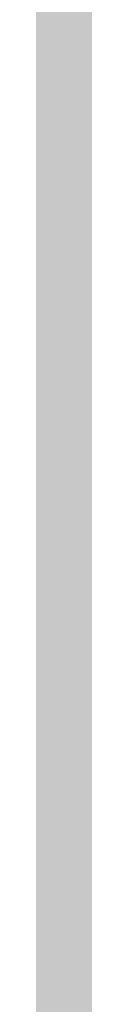
# Model space of a CAD drawing. Units: millimetres. Extents: x 0 to 2267, y 0 to 1823.
# Tile 41 of 256: x 1593.4369 to 1593.4507, y 1226.3857 to 1226.718. Entities that reach past the tile are written whole.
import ezdxf

# ---------------------------------------------------------------- set-up
doc = ezdxf.new("R2010")
doc.units = ezdxf.units.MM
doc.header["$MEASUREMENT"] = 0
doc.layers.add('M-HATC', color=252, linetype='Continuous', lineweight=18)

msp = doc.modelspace()

# ---------------------------------------------------------------- hatches: boundary and pattern name
at = {"layer": 'M-HATC'}
h = msp.add_hatch(color=256, dxfattribs=at)
h.dxf.hatch_style = 1
h.paths.add_polyline_path([(2055.77105, 1603.06204), (1381.08677, 1603.06204), (1381.08677, 1598.06204), (2055.77105, 1598.06204)])
h.paths.add_polyline_path([(2055.77105, 1598.06204), (1381.08677, 1598.06204), (1381.08677, 1593.06204), (2055.77105, 1593.06204)])
h.paths.add_polyline_path([(2051.30737, 1536.76088), (1385.55044, 1536.76088), (1385.55044, 1526.76088), (1387.55044, 1526.76088), (1388.53662, 1525.05276), (1385.33187, 1521.23348), (1385.33187, 1521.22256), (2050.25417, 1522.74913), (2048.32119, 1525.05276), (2049.30737, 1526.76088), (2051.30737, 1526.76088)])
edge = h.paths.add_edge_path()
edge.add_arc((1847.53451, 1379.14917), 135, 222.6030607, 222.8908505, ccw=False)
edge.add_line((1748.16629, 1287.76561), (1683.09212, 1287.76561))
edge.add_arc((1583.7239, 1379.14917), 135, 317.1091495, 317.3969393, ccw=False)
edge.add_arc((1678.9686, 1290.67067), 5, 222.89085, 317.10915, ccw=False)
edge.add_arc((1774.21331, 1379.14917), 135, 222.6030607, 222.8908505, ccw=False)
edge.add_line((1674.84509, 1287.76561), (1609.77092, 1287.76561))
edge.add_arc((1510.4027, 1379.14917), 135, 317.1091495, 317.3969393, ccw=False)
edge.add_arc((1605.6474, 1290.67067), 5, 222.89085, 317.10915, ccw=False)
edge.add_arc((1700.89211, 1379.14917), 135, 222.6030607, 222.8908505, ccw=False)
edge.add_line((1601.52388, 1287.76561), (1536.44972, 1287.76561))
edge.add_arc((1437.08149, 1379.14917), 135, 317.1091495, 317.3969393, ccw=False)
edge.add_arc((1532.3262, 1290.67067), 5, 222.89085, 317.10915, ccw=False)
edge.add_arc((1627.57091, 1379.14917), 135, 222.6030607, 222.8908505, ccw=False)
edge.add_line((1528.20268, 1287.76561), (1505.92891, 1287.76561))
edge.add_spline(control_points=[(1505.92891, 1287.76561), (1504.26224, 1287.76561), (1504.26224, 1282.76561), (1505.92891, 1282.76561)], knot_values=[0, 0, 0, 0, 5, 5, 5, 5], degree=3, periodic=0)
edge.add_line((1505.92891, 1282.76561), (1930.92891, 1282.76561))
edge.add_spline(control_points=[(1930.92891, 1282.76561), (1932.59557, 1282.76561), (1932.59557, 1287.76561), (1930.92891, 1287.76561)], knot_values=[0, 0, 0, 0, 5, 5, 5, 5], degree=3, periodic=0)
edge.add_line((1930.92891, 1287.76561), (1903.05573, 1287.76561))
edge.add_arc((1803.6875, 1379.14917), 135, 317.1091495, 317.3969393, ccw=False)
edge.add_arc((1898.93221, 1290.67067), 5, 222.89085, 317.10915, ccw=False)
edge.add_arc((1994.17691, 1379.14917), 135, 222.6030607, 222.8908505, ccw=False)
edge.add_line((1894.80869, 1287.76561), (1829.73452, 1287.76561))
edge.add_arc((1730.3663, 1379.14917), 135, 317.1091495, 317.3969393, ccw=False)
edge.add_arc((1825.61101, 1290.67067), 5, 222.89085, 317.10915, ccw=False)
edge.add_arc((1920.85571, 1379.14917), 135, 222.6030607, 222.8908505, ccw=False)
edge.add_line((1821.48749, 1287.76561), (1756.41332, 1287.76561))
edge.add_arc((1657.0451, 1379.14917), 135, 317.1091495, 317.3969393, ccw=False)
edge.add_arc((1752.28981, 1290.67067), 5, 222.89085, 317.10915, ccw=False)
edge = h.paths.add_edge_path()
edge.add_spline(control_points=[(1843.42891, 1227.24746), (1845.09557, 1227.24746), (1845.09557, 1232.24746), (1843.42891, 1232.24746)], knot_values=[0, 0, 0, 0, 5, 5, 5, 5], degree=3, periodic=0)
edge.add_line((1843.42891, 1232.24746), (1593.42891, 1232.24746))
edge.add_spline(control_points=[(1593.42891, 1232.24746), (1591.76224, 1232.24746), (1591.76224, 1227.24746), (1593.42891, 1227.24746)], knot_values=[0, 0, 0, 0, 5, 5, 5, 5], degree=3, periodic=0)
edge.add_line((1593.42891, 1227.24746), (1843.42891, 1227.24746))
h.paths.add_polyline_path([(1905.92891, 1127.41706), (1530.92891, 1127.41706, 0.414214), (1520.92891, 1117.41706), (1530.92891, 1117.41706), (1915.92891, 1117.41706, 0.414214)])
edge = h.paths.add_edge_path()
edge.add_arc((1397.08577, 1498.40775), 12.72993, 90.782146, 190.878706, ccw=False)
edge.add_line((1396.912, 1511.13649), (1428.00968, 1511.34875))
edge.add_line((1428.00968, 1511.34875), (1433.00968, 1511.34875))
edge.add_line((1433.00968, 1511.34875), (1434.439, 1511.34875))
edge.add_arc((1419.474, 1498.08041), 20, 41.560995, 74.082109)
edge.add_line((1424.95919, 1517.31353), (1399.93509, 1517.25608))
edge.add_spline(control_points=[(1399.93074, 1517.25607), (1399.88398, 1517.21312), (1399.8328, 1517.16893), (1399.77741, 1517.1236)], knot_values=[11.567499, 11.567499, 11.567499, 11.567499, 11.814249, 11.814249, 11.814249, 11.814249], degree=3, periodic=0)
edge.add_spline(control_points=[(1399.63279, 1517.00986), (1399.58305, 1516.97214), (1399.53072, 1516.93375), (1399.47591, 1516.89474)], knot_values=[11.167718, 11.167718, 11.167718, 11.167718, 11.365188, 11.365188, 11.365188, 11.365188], degree=3, periodic=0)
edge.add_spline(control_points=[(1399.33981, 1516.80007), (1399.15144, 1516.67185), (1398.93836, 1516.5377), (1398.70404, 1516.39942)], knot_values=[10.376405, 10.376405, 10.376405, 10.376405, 11.00994, 11.00994, 11.00994, 11.00994], degree=3, periodic=0)
edge.add_spline(control_points=[(1398.65716, 1516.37187), (1398.57885, 1516.32602), (1398.49825, 1516.27974), (1398.41549, 1516.23309)], knot_values=[10.125175, 10.125175, 10.125175, 10.125175, 10.334406, 10.334406, 10.334406, 10.334406], degree=3, periodic=0)
edge.add_spline(control_points=[(1398.26422, 1516.14874), (1398.19595, 1516.11107), (1398.12634, 1516.07319), (1398.05546, 1516.03513)], knot_values=[9.832246, 9.832246, 9.832246, 9.832246, 9.999658, 9.999658, 9.999658, 9.999658], degree=3, periodic=0)
edge.add_spline(control_points=[(1397.9987, 1516.00476), (1397.73115, 1515.86211), (1397.44602, 1515.71707), (1397.14664, 1515.57138)], knot_values=[9.161808, 9.161808, 9.161808, 9.161808, 9.787769, 9.787769, 9.787769, 9.787769], degree=3, periodic=0)
edge.add_spline(control_points=[(1397.14664, 1515.57138), (1396.84182, 1515.42305), (1396.52223, 1515.27404), (1396.1914, 1515.12621)], knot_values=[8.524455, 8.524455, 8.524455, 8.524455, 9.161808, 9.161808, 9.161808, 9.161808], degree=3, periodic=0)
edge.add_spline(control_points=[(1396.07771, 1515.07565), (1395.98538, 1515.03478), (1395.89222, 1514.99402), (1395.7983, 1514.9534)], knot_values=[8.275193, 8.275193, 8.275193, 8.275193, 8.451726, 8.451726, 8.451726, 8.451726], degree=3, periodic=0)
edge.add_spline(control_points=[(1395.60184, 1514.86912), (1395.49975, 1514.82568), (1395.39685, 1514.78244), (1395.29322, 1514.73944)], knot_values=[7.962917, 7.962917, 7.962917, 7.962917, 8.152764, 8.152764, 8.152764, 8.152764], degree=3, periodic=0)
edge.add_spline(control_points=[(1395.21158, 1514.70568), (1394.82779, 1514.5475), (1394.43452, 1514.39287), (1394.03645, 1514.24422)], knot_values=[7.21254, 7.21254, 7.21254, 7.21254, 7.913148, 7.913148, 7.913148, 7.913148], degree=3, periodic=0)
edge.add_spline(control_points=[(1394.03645, 1514.24422), (1393.70758, 1514.12142), (1393.37544, 1514.0027), (1393.04267, 1513.88945)], knot_values=[6.633733, 6.633733, 6.633733, 6.633733, 7.21254, 7.21254, 7.21254, 7.21254], degree=3, periodic=0)
edge.add_spline(control_points=[(1392.82142, 1513.81499), (1392.71978, 1513.78118), (1392.61815, 1513.74791), (1392.51658, 1513.71521)], knot_values=[6.328796, 6.328796, 6.328796, 6.328796, 6.505493, 6.505493, 6.505493, 6.505493], degree=3, periodic=0)
edge.add_spline(control_points=[(1392.51658, 1513.71521), (1392.31873, 1513.65151), (1392.12116, 1513.59001), (1391.92441, 1513.53098)], knot_values=[5.984605, 5.984605, 5.984605, 5.984605, 6.328796, 6.328796, 6.328796, 6.328796], degree=3, periodic=0)
edge.add_spline(control_points=[(1391.79155, 1513.49146), (1391.31215, 1513.35011), (1390.83842, 1513.22392), (1390.37844, 1513.11711)], knot_values=[5.066697, 5.066697, 5.066697, 5.066697, 5.907055, 5.907055, 5.907055, 5.907055], degree=3, periodic=0)
edge.add_spline(control_points=[(1390.37844, 1513.11711), (1390.17973, 1513.07097), (1389.98359, 1513.02845), (1389.79067, 1512.98988)], knot_values=[4.70367, 4.70367, 4.70367, 4.70367, 5.066695, 5.066695, 5.066695, 5.066695], degree=3, periodic=0)
edge.add_spline(control_points=[(1389.42203, 1512.92036), (1389.24588, 1512.88922), (1389.0729, 1512.86172), (1388.90364, 1512.83814)], knot_values=[4.130571, 4.130571, 4.130571, 4.130571, 4.469816, 4.469816, 4.469816, 4.469816], degree=3, periodic=0)
edge.add_spline(control_points=[(1388.90364, 1512.83814), (1388.59103, 1512.7946), (1388.29108, 1512.76444), (1388.00714, 1512.74941)], knot_values=[3.504031, 3.504031, 3.504031, 3.504031, 4.130571, 4.130571, 4.130571, 4.130571], degree=3, periodic=0)
edge.add_spline(control_points=[(1387.9356, 1512.74593), (1387.85378, 1512.74231), (1387.77334, 1512.73997), (1387.69435, 1512.73898)], knot_values=[3.268866, 3.268866, 3.268866, 3.268866, 3.451164, 3.451164, 3.451164, 3.451164], degree=3, periodic=0)
edge.add_spline(control_points=[(1387.33512, 1512.74426), (1387.20757, 1512.74991), (1387.08472, 1512.7597), (1386.96699, 1512.77385)], knot_values=[2.670686, 2.670686, 2.670686, 2.670686, 2.984, 2.984, 2.984, 2.984], degree=3, periodic=0)
edge.add_spline(control_points=[(1386.83274, 1512.79225), (1386.82093, 1512.79407), (1386.80917, 1512.79594), (1386.79747, 1512.79787)], knot_values=[2.516981, 2.516981, 2.516981, 2.516981, 2.549528, 2.549528, 2.549528, 2.549528], degree=3, periodic=0)
edge.add_spline(control_points=[(1386.45257, 1512.87348), (1386.42573, 1512.88105), (1386.39931, 1512.88895), (1386.3733, 1512.89719)], knot_values=[2.095869, 2.095869, 2.095869, 2.095869, 2.17941, 2.17941, 2.17941, 2.17941], degree=3, periodic=0)
edge.add_spline(control_points=[(1386.06911, 1513.01889), (1386.06338, 1513.02174), (1386.05768, 1513.02463), (1386.05201, 1513.02753)], knot_values=[1.72453, 1.72453, 1.72453, 1.72453, 1.745933, 1.745933, 1.745933, 1.745933], degree=3, periodic=0)
edge.add_arc((1399.474, 1498.08041), 20, 131.824322, 180)
edge.add_arc((1630.33362, 1505.54843), 250.97076, 181.7051759, 236.427975)
edge.add_arc((1605.33992, 1483.30441), 218.7822, 238.660829, 243.3496099)
edge.add_arc((1647.09105, 1510.35917), 262.89859, 183.1298361, 237.8534422, ccw=False)
h.paths.add_polyline_path([(1406.53685, 1391.96444, 0.149382), (1491.55061, 1296.44177, -0.129517)], flags=17)
edge = h.paths.add_edge_path()
edge.add_arc((2037.38381, 1498.08041), 20, 0, 48.265868)
edge.add_spline(control_points=[(2050.69731, 1513.00525), (2050.65121, 1512.98471), (2050.60338, 1512.96554), (2050.55388, 1512.94771)], knot_values=[1.835652, 1.835652, 1.835652, 1.835652, 2.000781, 2.000781, 2.000781, 2.000781], degree=3, periodic=0)
edge.add_spline(control_points=[(2050.46156, 1512.91661), (2050.479, 1512.9221), (2050.49625, 1512.92774), (2050.51332, 1512.93353)], knot_values=[2.045477, 2.045477, 2.045477, 2.045477, 2.101389, 2.101389, 2.101389, 2.101389], degree=3, periodic=0)
edge.add_spline(control_points=[(2050.12896, 1512.83416), (2050.19843, 1512.84734), (2050.26573, 1512.86233), (2050.33075, 1512.87919)], knot_values=[2.237629, 2.237629, 2.237629, 2.237629, 2.435841, 2.435841, 2.435841, 2.435841], degree=3, periodic=0)
edge.add_spline(control_points=[(2050.09463, 1512.82783), (2050.10613, 1512.82989), (2050.11757, 1512.832), (2050.12896, 1512.83416)], knot_values=[2.435841, 2.435841, 2.435841, 2.435841, 2.468321, 2.468321, 2.468321, 2.468321], degree=3, periodic=0)
edge.add_spline(control_points=[(2049.78433, 1512.78511), (2049.85521, 1512.79219), (2049.92435, 1512.80077), (2049.99166, 1512.81088)], knot_values=[2.563852, 2.563852, 2.563852, 2.563852, 2.748541, 2.748541, 2.748541, 2.748541], degree=3, periodic=0)
edge.add_spline(control_points=[(2049.4052, 1512.76169), (2049.5364, 1512.76526), (2049.66292, 1512.77299), (2049.78433, 1512.78511)], knot_values=[2.748541, 2.748541, 2.748541, 2.748541, 3.064882, 3.064882, 3.064882, 3.064882], degree=3, periodic=0)
edge.add_spline(control_points=[(2049.16976, 1512.75968), (2049.23364, 1512.7591), (2049.29654, 1512.7594), (2049.35844, 1512.7606)], knot_values=[3.102309, 3.102309, 3.102309, 3.102309, 3.2503, 3.2503, 3.2503, 3.2503], degree=3, periodic=0)
edge.add_spline(control_points=[(2048.85727, 1512.76911), (2048.96378, 1512.76378), (2049.068, 1512.76061), (2049.16976, 1512.75968)], knot_values=[3.2503, 3.2503, 3.2503, 3.2503, 3.486069, 3.486069, 3.486069, 3.486069], degree=3, periodic=0)
edge.add_spline(control_points=[(2048.69241, 1512.77892), (2048.3729, 1512.80093), (2048.0345, 1512.84106), (2047.68175, 1512.89697)], knot_values=[3.606429, 3.606429, 3.606429, 3.606429, 4.2989, 4.2989, 4.2989, 4.2989], degree=3, periodic=0)
edge.add_spline(control_points=[(2047.68175, 1512.89697), (2047.5458, 1512.91852), (2047.40772, 1512.94241), (2047.26776, 1512.96851)], knot_values=[4.2989, 4.2989, 4.2989, 4.2989, 4.565769, 4.565769, 4.565769, 4.565769], degree=3, periodic=0)
edge.add_spline(control_points=[(2047.26776, 1512.96851), (2047.14494, 1512.99141), (2047.02067, 1513.01601), (2046.89514, 1513.04223)], knot_values=[4.565769, 4.565769, 4.565769, 4.565769, 4.799971, 4.799971, 4.799971, 4.799971], degree=3, periodic=0)
edge.add_spline(control_points=[(2046.89514, 1513.04223), (2046.52865, 1513.11875), (2046.15135, 1513.20899), (2045.7676, 1513.31068)], knot_values=[4.799971, 4.799971, 4.799971, 4.799971, 5.483718, 5.483718, 5.483718, 5.483718], degree=3, periodic=0)
edge.add_spline(control_points=[(2045.7676, 1513.31068), (2045.3724, 1513.41539), (2044.97036, 1513.53225), (2044.56625, 1513.65876)], knot_values=[5.483718, 5.483718, 5.483718, 5.483718, 6.187866, 6.187866, 6.187866, 6.187866], degree=3, periodic=0)
edge.add_spline(control_points=[(2044.56625, 1513.65876), (2044.41491, 1513.70614), (2044.26329, 1513.75487), (2044.11163, 1513.80482)], knot_values=[6.187866, 6.187866, 6.187866, 6.187866, 6.451551, 6.451551, 6.451551, 6.451551], degree=3, periodic=0)
edge.add_spline(control_points=[(2044.11163, 1513.80482), (2043.99666, 1513.84269), (2043.88167, 1513.88126), (2043.76676, 1513.92048)], knot_values=[6.451551, 6.451551, 6.451551, 6.451551, 6.651434, 6.651434, 6.651434, 6.651434], degree=3, periodic=0)
edge.add_spline(control_points=[(2043.76676, 1513.92048), (2043.37157, 1514.05536), (2042.97738, 1514.19789), (2042.58863, 1514.34575)], knot_values=[6.651434, 6.651434, 6.651434, 6.651434, 7.338879, 7.338879, 7.338879, 7.338879], degree=3, periodic=0)
edge.add_spline(control_points=[(2042.58863, 1514.34575), (2042.16431, 1514.50715), (2041.74647, 1514.67491), (2041.34086, 1514.84603)], knot_values=[7.338879, 7.338879, 7.338879, 7.338879, 8.089209, 8.089209, 8.089209, 8.089209], degree=3, periodic=0)
edge.add_spline(control_points=[(2041.34086, 1514.84603), (2041.1028, 1514.94647), (2040.86896, 1515.04806), (2040.64049, 1515.1502)], knot_values=[8.089209, 8.089209, 8.089209, 8.089209, 8.529587, 8.529587, 8.529587, 8.529587], degree=3, periodic=0)
edge.add_spline(control_points=[(2040.50999, 1515.20887), (2040.08238, 1515.40218), (2039.67475, 1515.59705), (2039.29495, 1515.78939)], knot_values=[8.613818, 8.613818, 8.613818, 8.613818, 9.44571, 9.44571, 9.44571, 9.44571], degree=3, periodic=0)
edge.add_spline(control_points=[(2039.29495, 1515.78939), (2039.0618, 1515.90746), (2038.83914, 1516.02458), (2038.62878, 1516.1398)], knot_values=[9.44571, 9.44571, 9.44571, 9.44571, 9.956404, 9.956404, 9.956404, 9.956404], degree=3, periodic=0)
edge.add_spline(control_points=[(2038.62878, 1516.1398), (2038.51874, 1516.20007), (2038.41207, 1516.25982), (2038.30903, 1516.31891)], knot_values=[9.956404, 9.956404, 9.956404, 9.956404, 10.223542, 10.223542, 10.223542, 10.223542], degree=3, periodic=0)
edge.add_spline(control_points=[(2038.30903, 1516.31891), (2038.21377, 1516.37354), (2038.12161, 1516.42762), (2038.03275, 1516.48102)], knot_values=[10.223542, 10.223542, 10.223542, 10.223542, 10.47051, 10.47051, 10.47051, 10.47051], degree=3, periodic=0)
edge.add_spline(control_points=[(2038.03275, 1516.48102), (2037.78552, 1516.62961), (2037.56388, 1516.77304), (2037.37225, 1516.909)], knot_values=[10.47051, 10.47051, 10.47051, 10.47051, 11.15767, 11.15767, 11.15767, 11.15767], degree=3, periodic=0)
edge.add_spline(control_points=[(2037.37225, 1516.909), (2037.27893, 1516.9752), (2037.19274, 1517.03963), (2037.11417, 1517.10203)], knot_values=[11.15767, 11.15767, 11.15767, 11.15767, 11.49227, 11.49227, 11.49227, 11.49227], degree=3, periodic=0)
edge.add_spline(control_points=[(2036.85638, 1517.32585), (2036.91481, 1517.26923), (2036.98143, 1517.21027), (2037.05573, 1517.14922)], knot_values=[11.577341, 11.577341, 11.577341, 11.577341, 11.91035, 11.91035, 11.91035, 11.91035], degree=3, periodic=0)
edge.add_spline(control_points=[(2036.80739, 1517.37475), (2036.82301, 1517.35865), (2036.83935, 1517.34235), (2036.85638, 1517.32585)], knot_values=[11.91035, 11.91035, 11.91035, 11.91035, 12.007402, 12.007402, 12.007402, 12.007402], degree=3, periodic=0)
edge.add_spline(control_points=[(2036.70167, 1517.494), (2036.71042, 1517.48299), (2036.71958, 1517.47185), (2036.72913, 1517.4606)], knot_values=[12.184155, 12.184155, 12.184155, 12.184155, 12.255409, 12.255409, 12.255409, 12.255409], degree=3, periodic=0)
edge.add_spline(control_points=[(2036.6159, 1517.6205), (2036.61998, 1517.61304), (2036.6243, 1517.6055), (2036.62885, 1517.59789)], knot_values=[12.487913, 12.487913, 12.487913, 12.487913, 12.541035, 12.541035, 12.541035, 12.541035], degree=3, periodic=0)
edge.add_spline(control_points=[(2036.56349, 1517.78599), (2036.56372, 1517.77936), (2036.56423, 1517.77264), (2036.56502, 1517.76582)], knot_values=[12.911761, 12.911761, 12.911761, 12.911761, 12.968286, 12.968286, 12.968286, 12.968286], degree=3, periodic=0)
edge.add_spline(control_points=[(2036.61663, 1517.93042), (2036.61248, 1517.92586), (2036.60857, 1517.92121), (2036.60491, 1517.91648)], knot_values=[13.382527, 13.382527, 13.382527, 13.382527, 13.433791, 13.433791, 13.433791, 13.433791], degree=3, periodic=0)
edge.add_spline(control_points=[(2036.74902, 1518.01695), (2036.73613, 1518.0116), (2036.72393, 1518.00601), (2036.71242, 1518.00018)], knot_values=[13.726299, 13.726299, 13.726299, 13.726299, 13.809928, 13.809928, 13.809928, 13.809928], degree=3, periodic=0)
edge.add_spline(control_points=[(2036.86043, 1518.05285), (2036.83863, 1518.04743), (2036.81809, 1518.04156), (2036.79879, 1518.03526)], knot_values=[13.910887, 13.910887, 13.910887, 13.910887, 14.02153, 14.02153, 14.02153, 14.02153], degree=3, periodic=0)
edge.add_line((2036.96387, 1518.08041), (2032.38381, 1518.08041))
edge.add_line((2032.38381, 1518.08041), (2027.38381, 1518.08041))
edge.add_line((2027.38381, 1518.08041), (2022.38381, 1518.08041))
edge.add_line((2022.38381, 1518.08041), (2017.38381, 1518.08041))
edge.add_arc((2017.38381, 1498.08041), 20, 90, 138.439005)
edge.add_line((2002.41881, 1511.34875), (2003.84813, 1511.34875))
edge.add_line((2003.84813, 1511.34875), (2008.84813, 1511.34875))
edge.add_line((2008.84813, 1511.34875), (2039.77204, 1511.13768))
edge.add_arc((2039.77204, 1498.40775), 12.72993, -10.878706, 90, ccw=False)
edge.add_arc((1789.76676, 1510.35917), 262.89859, 302.1465578, 356.8701639, ccw=False)
edge.add_arc((1831.51789, 1483.30441), 218.7822, 296.6503901, 301.339171)
edge.add_arc((1806.52419, 1505.54843), 250.97076, 303.572025, 358.2948241)
h.paths.add_polyline_path([(2030.32096, 1391.96444, -0.129517), (1945.3072, 1296.44177, 0.149382)], flags=17)
edge = h.paths.add_edge_path()
edge.add_spline(control_points=[(2037.2464, 1518.08209), (2037.28977, 1518.08098), (2037.33555, 1518.08041), (2037.3838, 1518.08041)], knot_values=[0.000012, 0.000012, 0.000012, 0.000012, 0.144754, 0.144754, 0.144754, 0.144754], degree=3, periodic=0)
edge.add_line((2037.33571, 1518.08041), (2037.00963, 1518.08041))
edge.add_spline(control_points=[(2037.00963, 1518.08041), (2036.98217, 1518.07678), (2036.95605, 1518.07266), (2036.93124, 1518.06808)], knot_values=[14.13465, 14.13465, 14.13465, 14.13465, 14.247197, 14.247197, 14.247197, 14.247197], degree=3, periodic=0)
edge.add_spline(control_points=[(2036.93124, 1518.06808), (2036.92764, 1518.06741), (2036.92407, 1518.06674), (2036.92053, 1518.06605)], knot_values=[14.118315, 14.118315, 14.118315, 14.118315, 14.13465, 14.13465, 14.13465, 14.13465], degree=3, periodic=0)
edge.add_spline(control_points=[(2036.92053, 1518.06605), (2036.9118, 1518.06436), (2036.90323, 1518.06262), (2036.89484, 1518.06081)], knot_values=[14.078086, 14.078086, 14.078086, 14.078086, 14.118315, 14.118315, 14.118315, 14.118315], degree=3, periodic=0)
edge.add_spline(control_points=[(2036.89484, 1518.06081), (2036.88304, 1518.05827), (2036.87157, 1518.05562), (2036.86043, 1518.05285)], knot_values=[14.02153, 14.02153, 14.02153, 14.02153, 14.078086, 14.078086, 14.078086, 14.078086], degree=3, periodic=0)
edge.add_spline(control_points=[(2036.86043, 1518.05285), (2036.83863, 1518.04743), (2036.81809, 1518.04156), (2036.79879, 1518.03526)], knot_values=[13.910887, 13.910887, 13.910887, 13.910887, 14.02153, 14.02153, 14.02153, 14.02153], degree=3, periodic=0)
edge.add_spline(control_points=[(2036.79879, 1518.03526), (2036.79809, 1518.03504), (2036.7974, 1518.03481), (2036.79671, 1518.03458)], knot_values=[13.906906, 13.906906, 13.906906, 13.906906, 13.910887, 13.910887, 13.910887, 13.910887], degree=3, periodic=0)
edge.add_spline(control_points=[(2036.79671, 1518.03458), (2036.78819, 1518.03178), (2036.77991, 1518.02888), (2036.77187, 1518.02591)], knot_values=[13.857826, 13.857826, 13.857826, 13.857826, 13.906906, 13.906906, 13.906906, 13.906906], degree=3, periodic=0)
edge.add_spline(control_points=[(2036.77187, 1518.02591), (2036.76402, 1518.023), (2036.75641, 1518.02002), (2036.74902, 1518.01695)], knot_values=[13.809928, 13.809928, 13.809928, 13.809928, 13.857826, 13.857826, 13.857826, 13.857826], degree=3, periodic=0)
edge.add_spline(control_points=[(2036.74902, 1518.01695), (2036.73613, 1518.0116), (2036.72393, 1518.00601), (2036.71242, 1518.00018)], knot_values=[13.726299, 13.726299, 13.726299, 13.726299, 13.809928, 13.809928, 13.809928, 13.809928], degree=3, periodic=0)
edge.add_spline(control_points=[(2036.71242, 1518.00018), (2036.71211, 1518.00002), (2036.71179, 1517.99986), (2036.71147, 1517.99969)], knot_values=[13.723993, 13.723993, 13.723993, 13.723993, 13.726299, 13.726299, 13.726299, 13.726299], degree=3, periodic=0)
edge.add_spline(control_points=[(2036.71147, 1517.99969), (2036.70634, 1517.99708), (2036.70134, 1517.99441), (2036.69648, 1517.9917)], knot_values=[13.686536, 13.686536, 13.686536, 13.686536, 13.723993, 13.723993, 13.723993, 13.723993], degree=3, periodic=0)
edge.add_spline(control_points=[(2036.69648, 1517.9917), (2036.6919, 1517.98914), (2036.68744, 1517.98654), (2036.6831, 1517.9839)], knot_values=[13.651251, 13.651251, 13.651251, 13.651251, 13.686536, 13.686536, 13.686536, 13.686536], degree=3, periodic=0)
edge.add_spline(control_points=[(2036.6831, 1517.9839), (2036.67641, 1517.97983), (2036.67001, 1517.97566), (2036.6639, 1517.97139)], knot_values=[13.596804, 13.596804, 13.596804, 13.596804, 13.651251, 13.651251, 13.651251, 13.651251], degree=3, periodic=0)
edge.add_spline(control_points=[(2036.6639, 1517.97139), (2036.66358, 1517.97117), (2036.66326, 1517.97094), (2036.66294, 1517.97072)], knot_values=[13.593956, 13.593956, 13.593956, 13.593956, 13.596804, 13.596804, 13.596804, 13.596804], degree=3, periodic=0)
edge.add_spline(control_points=[(2036.66294, 1517.97072), (2036.6603, 1517.96886), (2036.65771, 1517.96698), (2036.65518, 1517.96509)], knot_values=[13.570322, 13.570322, 13.570322, 13.570322, 13.593956, 13.593956, 13.593956, 13.593956], degree=3, periodic=0)
edge.add_spline(control_points=[(2036.65518, 1517.96509), (2036.65251, 1517.9631), (2036.64991, 1517.96108), (2036.64737, 1517.95905)], knot_values=[13.545477, 13.545477, 13.545477, 13.545477, 13.570322, 13.570322, 13.570322, 13.570322], degree=3, periodic=0)
edge.add_spline(control_points=[(2036.64737, 1517.95905), (2036.64721, 1517.95892), (2036.64705, 1517.9588), (2036.64689, 1517.95867)], knot_values=[13.543931, 13.543931, 13.543931, 13.543931, 13.545477, 13.545477, 13.545477, 13.545477], degree=3, periodic=0)
edge.add_spline(control_points=[(2036.64689, 1517.95867), (2036.64121, 1517.95411), (2036.63582, 1517.94945), (2036.63073, 1517.94468)], knot_values=[13.488237, 13.488237, 13.488237, 13.488237, 13.543931, 13.543931, 13.543931, 13.543931], degree=3, periodic=0)
edge.add_spline(control_points=[(2036.63073, 1517.94468), (2036.62817, 1517.94229), (2036.62569, 1517.93988), (2036.62329, 1517.93744)], knot_values=[13.460307, 13.460307, 13.460307, 13.460307, 13.488237, 13.488237, 13.488237, 13.488237], degree=3, periodic=0)
edge.add_spline(control_points=[(2036.62329, 1517.93744), (2036.62151, 1517.93564), (2036.61978, 1517.93383), (2036.61809, 1517.932)], knot_values=[13.439712, 13.439712, 13.439712, 13.439712, 13.460307, 13.460307, 13.460307, 13.460307], degree=3, periodic=0)
edge.add_spline(control_points=[(2036.61809, 1517.932), (2036.6176, 1517.93147), (2036.61711, 1517.93095), (2036.61663, 1517.93042)], knot_values=[13.433791, 13.433791, 13.433791, 13.433791, 13.439712, 13.439712, 13.439712, 13.439712], degree=3, periodic=0)
edge.add_spline(control_points=[(2036.61663, 1517.93042), (2036.61248, 1517.92586), (2036.60857, 1517.92121), (2036.60491, 1517.91648)], knot_values=[13.382527, 13.382527, 13.382527, 13.382527, 13.433791, 13.433791, 13.433791, 13.433791], degree=3, periodic=0)
edge.add_spline(control_points=[(2036.60491, 1517.91648), (2036.60258, 1517.91347), (2036.60036, 1517.91044), (2036.59824, 1517.90737)], knot_values=[13.350017, 13.350017, 13.350017, 13.350017, 13.382527, 13.382527, 13.382527, 13.382527], degree=3, periodic=0)
edge.add_spline(control_points=[(2036.59824, 1517.90737), (2036.59718, 1517.90585), (2036.59616, 1517.90433), (2036.59515, 1517.90279)], knot_values=[13.333922, 13.333922, 13.333922, 13.333922, 13.350017, 13.350017, 13.350017, 13.350017], degree=3, periodic=0)
edge.add_spline(control_points=[(2036.59515, 1517.90279), (2036.59452, 1517.90183), (2036.5939, 1517.90086), (2036.59329, 1517.89989)], knot_values=[13.323828, 13.323828, 13.323828, 13.323828, 13.333922, 13.333922, 13.333922, 13.333922], degree=3, periodic=0)
edge.add_spline(control_points=[(2036.59329, 1517.89989), (2036.59049, 1517.89545), (2036.5879, 1517.89094), (2036.5855, 1517.88637)], knot_values=[13.277545, 13.277545, 13.277545, 13.277545, 13.323828, 13.323828, 13.323828, 13.323828], degree=3, periodic=0)
edge.add_spline(control_points=[(2036.5855, 1517.88637), (2036.58355, 1517.88267), (2036.58174, 1517.87892), (2036.58006, 1517.87513)], knot_values=[13.240119, 13.240119, 13.240119, 13.240119, 13.277545, 13.277545, 13.277545, 13.277545], degree=3, periodic=0)
edge.add_spline(control_points=[(2036.58006, 1517.87513), (2036.57952, 1517.87393), (2036.579, 1517.87272), (2036.57849, 1517.87151)], knot_values=[13.228211, 13.228211, 13.228211, 13.228211, 13.240119, 13.240119, 13.240119, 13.240119], degree=3, periodic=0)
edge.add_spline(control_points=[(2036.57849, 1517.87151), (2036.57796, 1517.87023), (2036.57744, 1517.86896), (2036.57693, 1517.86767)], knot_values=[13.215717, 13.215717, 13.215717, 13.215717, 13.228211, 13.228211, 13.228211, 13.228211], degree=3, periodic=0)
edge.add_spline(control_points=[(2036.57693, 1517.86767), (2036.57548, 1517.86399), (2036.57414, 1517.86027), (2036.57293, 1517.85651)], knot_values=[13.179847, 13.179847, 13.179847, 13.179847, 13.215717, 13.215717, 13.215717, 13.215717], degree=3, periodic=0)
edge.add_spline(control_points=[(2036.57293, 1517.85651), (2036.5713, 1517.8515), (2036.56989, 1517.84641), (2036.56868, 1517.84126)], knot_values=[13.132017, 13.132017, 13.132017, 13.132017, 13.179847, 13.179847, 13.179847, 13.179847], degree=3, periodic=0)
edge.add_spline(control_points=[(2036.56868, 1517.84126), (2036.56844, 1517.84023), (2036.56821, 1517.8392), (2036.56798, 1517.83817)], knot_values=[13.122482, 13.122482, 13.122482, 13.122482, 13.132017, 13.132017, 13.132017, 13.132017], degree=3, periodic=0)
edge.add_spline(control_points=[(2036.56798, 1517.83817), (2036.56758, 1517.83634), (2036.56721, 1517.8345), (2036.56687, 1517.83266)], knot_values=[13.105592, 13.105592, 13.105592, 13.105592, 13.122482, 13.122482, 13.122482, 13.122482], degree=3, periodic=0)
edge.add_spline(control_points=[(2036.56687, 1517.83266), (2036.56622, 1517.82921), (2036.56567, 1517.82574), (2036.5652, 1517.82223)], knot_values=[13.074063, 13.074063, 13.074063, 13.074063, 13.105592, 13.105592, 13.105592, 13.105592], degree=3, periodic=0)
edge.add_spline(control_points=[(2036.5652, 1517.82223), (2036.5652, 1517.82223), (2036.5652, 1517.82223), (2036.5652, 1517.82223)], knot_values=[13.074043, 13.074043, 13.074043, 13.074043, 13.074063, 13.074063, 13.074063, 13.074063], degree=3, periodic=0)
edge.add_spline(control_points=[(2036.5652, 1517.82223), (2036.56443, 1517.81643), (2036.5639, 1517.81055), (2036.56361, 1517.8046)], knot_values=[13.021884, 13.021884, 13.021884, 13.021884, 13.074043, 13.074043, 13.074043, 13.074043], degree=3, periodic=0)
edge.add_spline(control_points=[(2036.56361, 1517.8046), (2036.56358, 1517.80401), (2036.56356, 1517.80342), (2036.56353, 1517.80283)], knot_values=[13.01674, 13.01674, 13.01674, 13.01674, 13.021884, 13.021884, 13.021884, 13.021884], degree=3, periodic=0)
edge.add_spline(control_points=[(2036.56353, 1517.80283), (2036.56344, 1517.80051), (2036.56338, 1517.79817), (2036.56336, 1517.79582)], knot_values=[12.996438, 12.996438, 12.996438, 12.996438, 13.01674, 13.01674, 13.01674, 13.01674], degree=3, periodic=0)
edge.add_spline(control_points=[(2036.56336, 1517.79582), (2036.56334, 1517.79257), (2036.56338, 1517.78929), (2036.56349, 1517.78599)], knot_values=[12.968286, 12.968286, 12.968286, 12.968286, 12.996438, 12.996438, 12.996438, 12.996438], degree=3, periodic=0)
edge.add_spline(control_points=[(2036.56349, 1517.78599), (2036.56372, 1517.77936), (2036.56423, 1517.77264), (2036.56502, 1517.76582)], knot_values=[12.911761, 12.911761, 12.911761, 12.911761, 12.968286, 12.968286, 12.968286, 12.968286], degree=3, periodic=0)
edge.add_spline(control_points=[(2036.56502, 1517.76582), (2036.56503, 1517.76573), (2036.56504, 1517.76564), (2036.56505, 1517.76555)], knot_values=[12.911017, 12.911017, 12.911017, 12.911017, 12.911761, 12.911761, 12.911761, 12.911761], degree=3, periodic=0)
edge.add_spline(control_points=[(2036.56505, 1517.76555), (2036.56541, 1517.76245), (2036.56583, 1517.75933), (2036.56631, 1517.75619)], knot_values=[12.88528, 12.88528, 12.88528, 12.88528, 12.911017, 12.911017, 12.911017, 12.911017], degree=3, periodic=0)
edge.add_spline(control_points=[(2036.56631, 1517.75619), (2036.56673, 1517.75341), (2036.5672, 1517.75062), (2036.56771, 1517.74782)], knot_values=[12.862519, 12.862519, 12.862519, 12.862519, 12.88528, 12.88528, 12.88528, 12.88528], degree=3, periodic=0)
edge.add_spline(control_points=[(2036.56771, 1517.74782), (2036.56779, 1517.74737), (2036.56788, 1517.74692), (2036.56796, 1517.74647)], knot_values=[12.858885, 12.858885, 12.858885, 12.858885, 12.862519, 12.862519, 12.862519, 12.862519], degree=3, periodic=0)
edge.add_spline(control_points=[(2036.56796, 1517.74647), (2036.5692, 1517.73986), (2036.57069, 1517.73316), (2036.57243, 1517.72638)], knot_values=[12.8053, 12.8053, 12.8053, 12.8053, 12.858885, 12.858885, 12.858885, 12.858885], degree=3, periodic=0)
edge.add_spline(control_points=[(2036.57243, 1517.72638), (2036.5734, 1517.72257), (2036.57446, 1517.71874), (2036.57559, 1517.71488)], knot_values=[12.775176, 12.775176, 12.775176, 12.775176, 12.8053, 12.8053, 12.8053, 12.8053], degree=3, periodic=0)
edge.add_spline(control_points=[(2036.57559, 1517.71488), (2036.57628, 1517.71252), (2036.577, 1517.71015), (2036.57775, 1517.70778)], knot_values=[12.756759, 12.756759, 12.756759, 12.756759, 12.775176, 12.775176, 12.775176, 12.775176], degree=3, periodic=0)
edge.add_spline(control_points=[(2036.57775, 1517.70778), (2036.57808, 1517.70674), (2036.57841, 1517.7057), (2036.57875, 1517.70466)], knot_values=[12.748742, 12.748742, 12.748742, 12.748742, 12.756759, 12.756759, 12.756759, 12.756759], degree=3, periodic=0)
edge.add_spline(control_points=[(2036.57875, 1517.70466), (2036.58082, 1517.6983), (2036.58309, 1517.69187), (2036.58557, 1517.68537)], knot_values=[12.69959, 12.69959, 12.69959, 12.69959, 12.748742, 12.748742, 12.748742, 12.748742], degree=3, periodic=0)
edge.add_spline(control_points=[(2036.58557, 1517.68537), (2036.58762, 1517.68001), (2036.5898, 1517.6746), (2036.59213, 1517.66916)], knot_values=[12.659038, 12.659038, 12.659038, 12.659038, 12.69959, 12.69959, 12.69959, 12.69959], degree=3, periodic=0)
edge.add_spline(control_points=[(2036.59213, 1517.66916), (2036.59397, 1517.66482), (2036.59591, 1517.66047), (2036.59793, 1517.65608)], knot_values=[12.626806, 12.626806, 12.626806, 12.626806, 12.659038, 12.659038, 12.659038, 12.659038], degree=3, periodic=0)
edge.add_spline(control_points=[(2036.59793, 1517.65608), (2036.59839, 1517.65507), (2036.59886, 1517.65406), (2036.59934, 1517.65305)], knot_values=[12.619394, 12.619394, 12.619394, 12.619394, 12.626806, 12.626806, 12.626806, 12.626806], degree=3, periodic=0)
edge.add_spline(control_points=[(2036.59934, 1517.65305), (2036.60435, 1517.64236), (2036.60987, 1517.63151), (2036.61589, 1517.6205)], knot_values=[12.541039, 12.541039, 12.541039, 12.541039, 12.619394, 12.619394, 12.619394, 12.619394], degree=3, periodic=0)
edge.add_spline(control_points=[(2036.61589, 1517.6205), (2036.61589, 1517.6205), (2036.6159, 1517.6205), (2036.6159, 1517.6205)], knot_values=[12.541035, 12.541035, 12.541035, 12.541035, 12.541039, 12.541039, 12.541039, 12.541039], degree=3, periodic=0)
edge.add_spline(control_points=[(2036.6159, 1517.6205), (2036.61998, 1517.61304), (2036.6243, 1517.6055), (2036.62885, 1517.59789)], knot_values=[12.487913, 12.487913, 12.487913, 12.487913, 12.541035, 12.541035, 12.541035, 12.541035], degree=3, periodic=0)
edge.add_spline(control_points=[(2036.62885, 1517.59789), (2036.63261, 1517.5916), (2036.63653, 1517.58526), (2036.64061, 1517.57888)], knot_values=[12.443982, 12.443982, 12.443982, 12.443982, 12.487913, 12.487913, 12.487913, 12.487913], degree=3, periodic=0)
edge.add_spline(control_points=[(2036.64061, 1517.57888), (2036.64144, 1517.57757), (2036.64228, 1517.57626), (2036.64313, 1517.57495)], knot_values=[12.434996, 12.434996, 12.434996, 12.434996, 12.443982, 12.443982, 12.443982, 12.443982], degree=3, periodic=0)
edge.add_spline(control_points=[(2036.64313, 1517.57495), (2036.65306, 1517.55958), (2036.66389, 1517.54394), (2036.6756, 1517.52803)], knot_values=[12.329647, 12.329647, 12.329647, 12.329647, 12.434996, 12.434996, 12.434996, 12.434996], degree=3, periodic=0)
edge.add_spline(control_points=[(2036.6756, 1517.52803), (2036.68385, 1517.51682), (2036.69254, 1517.50548), (2036.70167, 1517.494)], knot_values=[12.255409, 12.255409, 12.255409, 12.255409, 12.329647, 12.329647, 12.329647, 12.329647], degree=3, periodic=0)
edge.add_spline(control_points=[(2036.70167, 1517.494), (2036.71042, 1517.48299), (2036.71958, 1517.47185), (2036.72913, 1517.4606)], knot_values=[12.184155, 12.184155, 12.184155, 12.184155, 12.255409, 12.255409, 12.255409, 12.255409], degree=3, periodic=0)
edge.add_spline(control_points=[(2036.72913, 1517.4606), (2036.74363, 1517.44352), (2036.75904, 1517.42617), (2036.77534, 1517.40855)], knot_values=[12.075961, 12.075961, 12.075961, 12.075961, 12.184155, 12.184155, 12.184155, 12.184155], degree=3, periodic=0)
edge.add_spline(control_points=[(2036.77534, 1517.40855), (2036.77631, 1517.4075), (2036.77729, 1517.40645), (2036.77827, 1517.40539)], knot_values=[12.069502, 12.069502, 12.069502, 12.069502, 12.075961, 12.075961, 12.075961, 12.075961], degree=3, periodic=0)
edge.add_spline(control_points=[(2036.77827, 1517.40539), (2036.78768, 1517.39526), (2036.79739, 1517.38505), (2036.80739, 1517.37475)], knot_values=[12.007402, 12.007402, 12.007402, 12.007402, 12.069502, 12.069502, 12.069502, 12.069502], degree=3, periodic=0)
edge.add_spline(control_points=[(2036.80739, 1517.37475), (2036.82301, 1517.35865), (2036.83935, 1517.34235), (2036.85638, 1517.32585)], knot_values=[11.91035, 11.91035, 11.91035, 11.91035, 12.007402, 12.007402, 12.007402, 12.007402], degree=3, periodic=0)
edge.add_spline(control_points=[(2036.85638, 1517.32585), (2036.91481, 1517.26923), (2036.98143, 1517.21027), (2037.05573, 1517.14922)], knot_values=[11.577341, 11.577341, 11.577341, 11.577341, 11.91035, 11.91035, 11.91035, 11.91035], degree=3, periodic=0)
edge.add_spline(control_points=[(2037.05573, 1517.14922), (2037.07471, 1517.13362), (2037.0942, 1517.11789), (2037.11417, 1517.10203)], knot_values=[11.49227, 11.49227, 11.49227, 11.49227, 11.577341, 11.577341, 11.577341, 11.577341], degree=3, periodic=0)
edge.add_spline(control_points=[(2037.11417, 1517.10203), (2037.19274, 1517.03963), (2037.27893, 1516.9752), (2037.37225, 1516.909)], knot_values=[11.15767, 11.15767, 11.15767, 11.15767, 11.49227, 11.49227, 11.49227, 11.49227], degree=3, periodic=0)
edge.add_spline(control_points=[(2037.37225, 1516.909), (2037.56388, 1516.77304), (2037.78552, 1516.62961), (2038.03275, 1516.48102)], knot_values=[10.47051, 10.47051, 10.47051, 10.47051, 11.15767, 11.15767, 11.15767, 11.15767], degree=3, periodic=0)
edge.add_spline(control_points=[(2038.03275, 1516.48102), (2038.12161, 1516.42762), (2038.21377, 1516.37354), (2038.30903, 1516.31891)], knot_values=[10.223542, 10.223542, 10.223542, 10.223542, 10.47051, 10.47051, 10.47051, 10.47051], degree=3, periodic=0)
edge.add_spline(control_points=[(2038.30903, 1516.31891), (2038.41207, 1516.25982), (2038.51874, 1516.20007), (2038.62878, 1516.1398)], knot_values=[9.956404, 9.956404, 9.956404, 9.956404, 10.223542, 10.223542, 10.223542, 10.223542], degree=3, periodic=0)
edge.add_spline(control_points=[(2038.62878, 1516.1398), (2038.83914, 1516.02458), (2039.0618, 1515.90746), (2039.29495, 1515.78939)], knot_values=[9.44571, 9.44571, 9.44571, 9.44571, 9.956404, 9.956404, 9.956404, 9.956404], degree=3, periodic=0)
edge.add_spline(control_points=[(2039.29495, 1515.78939), (2039.67475, 1515.59705), (2040.08238, 1515.40218), (2040.50999, 1515.20887)], knot_values=[8.613818, 8.613818, 8.613818, 8.613818, 9.44571, 9.44571, 9.44571, 9.44571], degree=3, periodic=0)
edge.add_spline(control_points=[(2040.50999, 1515.20887), (2040.55329, 1515.1893), (2040.59679, 1515.16974), (2040.64049, 1515.1502)], knot_values=[8.529587, 8.529587, 8.529587, 8.529587, 8.613818, 8.613818, 8.613818, 8.613818], degree=3, periodic=0)
edge.add_spline(control_points=[(2040.64049, 1515.1502), (2040.86896, 1515.04806), (2041.1028, 1514.94647), (2041.34086, 1514.84603)], knot_values=[8.089209, 8.089209, 8.089209, 8.089209, 8.529587, 8.529587, 8.529587, 8.529587], degree=3, periodic=0)
edge.add_spline(control_points=[(2041.34086, 1514.84603), (2041.74647, 1514.67491), (2042.16431, 1514.50715), (2042.58863, 1514.34575)], knot_values=[7.338879, 7.338879, 7.338879, 7.338879, 8.089209, 8.089209, 8.089209, 8.089209], degree=3, periodic=0)
edge.add_spline(control_points=[(2042.58863, 1514.34575), (2042.97738, 1514.19789), (2043.37157, 1514.05536), (2043.76676, 1513.92048)], knot_values=[6.651434, 6.651434, 6.651434, 6.651434, 7.338879, 7.338879, 7.338879, 7.338879], degree=3, periodic=0)
edge.add_spline(control_points=[(2043.76676, 1513.92048), (2043.88167, 1513.88126), (2043.99666, 1513.84269), (2044.11163, 1513.80482)], knot_values=[6.451551, 6.451551, 6.451551, 6.451551, 6.651434, 6.651434, 6.651434, 6.651434], degree=3, periodic=0)
edge.add_spline(control_points=[(2044.11163, 1513.80482), (2044.26329, 1513.75487), (2044.41491, 1513.70614), (2044.56625, 1513.65876)], knot_values=[6.187866, 6.187866, 6.187866, 6.187866, 6.451551, 6.451551, 6.451551, 6.451551], degree=3, periodic=0)
edge.add_spline(control_points=[(2044.56625, 1513.65876), (2044.97036, 1513.53225), (2045.3724, 1513.41539), (2045.7676, 1513.31068)], knot_values=[5.483718, 5.483718, 5.483718, 5.483718, 6.187866, 6.187866, 6.187866, 6.187866], degree=3, periodic=0)
edge.add_spline(control_points=[(2045.7676, 1513.31068), (2046.15135, 1513.20899), (2046.52865, 1513.11875), (2046.89514, 1513.04223)], knot_values=[4.799971, 4.799971, 4.799971, 4.799971, 5.483718, 5.483718, 5.483718, 5.483718], degree=3, periodic=0)
edge.add_spline(control_points=[(2046.89514, 1513.04223), (2047.02067, 1513.01601), (2047.14494, 1512.99141), (2047.26776, 1512.96851)], knot_values=[4.565769, 4.565769, 4.565769, 4.565769, 4.799971, 4.799971, 4.799971, 4.799971], degree=3, periodic=0)
edge.add_spline(control_points=[(2047.26776, 1512.96851), (2047.40772, 1512.94241), (2047.5458, 1512.91852), (2047.68175, 1512.89697)], knot_values=[4.2989, 4.2989, 4.2989, 4.2989, 4.565769, 4.565769, 4.565769, 4.565769], degree=3, periodic=0)
edge.add_spline(control_points=[(2047.68175, 1512.89697), (2048.0345, 1512.84106), (2048.3729, 1512.80093), (2048.69241, 1512.77892)], knot_values=[3.606429, 3.606429, 3.606429, 3.606429, 4.2989, 4.2989, 4.2989, 4.2989], degree=3, periodic=0)
edge.add_spline(control_points=[(2048.69241, 1512.77892), (2048.74794, 1512.7751), (2048.8029, 1512.77182), (2048.85727, 1512.76911)], knot_values=[3.486069, 3.486069, 3.486069, 3.486069, 3.606429, 3.606429, 3.606429, 3.606429], degree=3, periodic=0)
edge.add_spline(control_points=[(2048.85727, 1512.76911), (2048.96378, 1512.76378), (2049.068, 1512.76061), (2049.16976, 1512.75968)], knot_values=[3.2503, 3.2503, 3.2503, 3.2503, 3.486069, 3.486069, 3.486069, 3.486069], degree=3, periodic=0)
edge.add_spline(control_points=[(2049.16976, 1512.75968), (2049.23364, 1512.7591), (2049.29654, 1512.7594), (2049.35844, 1512.7606)], knot_values=[3.102309, 3.102309, 3.102309, 3.102309, 3.2503, 3.2503, 3.2503, 3.2503], degree=3, periodic=0)
edge.add_spline(control_points=[(2049.35844, 1512.7606), (2049.37409, 1512.76091), (2049.38968, 1512.76127), (2049.4052, 1512.76169)], knot_values=[3.064882, 3.064882, 3.064882, 3.064882, 3.102309, 3.102309, 3.102309, 3.102309], degree=3, periodic=0)
edge.add_spline(control_points=[(2049.4052, 1512.76169), (2049.5364, 1512.76526), (2049.66292, 1512.77299), (2049.78433, 1512.78511)], knot_values=[2.748541, 2.748541, 2.748541, 2.748541, 3.064882, 3.064882, 3.064882, 3.064882], degree=3, periodic=0)
edge.add_spline(control_points=[(2049.78433, 1512.78511), (2049.85521, 1512.79219), (2049.92435, 1512.80077), (2049.99166, 1512.81088)], knot_values=[2.563852, 2.563852, 2.563852, 2.563852, 2.748541, 2.748541, 2.748541, 2.748541], degree=3, periodic=0)
edge.add_spline(control_points=[(2049.99166, 1512.81088), (2050.02648, 1512.81612), (2050.0608, 1512.82177), (2050.09463, 1512.82783)], knot_values=[2.468321, 2.468321, 2.468321, 2.468321, 2.563852, 2.563852, 2.563852, 2.563852], degree=3, periodic=0)
edge.add_spline(control_points=[(2050.09463, 1512.82783), (2050.10613, 1512.82989), (2050.11757, 1512.832), (2050.12896, 1512.83416)], knot_values=[2.435841, 2.435841, 2.435841, 2.435841, 2.468321, 2.468321, 2.468321, 2.468321], degree=3, periodic=0)
edge.add_spline(control_points=[(2050.12896, 1512.83416), (2050.19843, 1512.84734), (2050.26573, 1512.86233), (2050.33075, 1512.87919)], knot_values=[2.237629, 2.237629, 2.237629, 2.237629, 2.435841, 2.435841, 2.435841, 2.435841], degree=3, periodic=0)
edge.add_spline(control_points=[(2050.33075, 1512.87919), (2050.37544, 1512.89077), (2050.41906, 1512.90324), (2050.46156, 1512.91661)], knot_values=[2.101389, 2.101389, 2.101389, 2.101389, 2.237629, 2.237629, 2.237629, 2.237629], degree=3, periodic=0)
edge.add_spline(control_points=[(2050.46156, 1512.91661), (2050.479, 1512.9221), (2050.49625, 1512.92774), (2050.51332, 1512.93353)], knot_values=[2.045477, 2.045477, 2.045477, 2.045477, 2.101389, 2.101389, 2.101389, 2.101389], degree=3, periodic=0)
edge.add_spline(control_points=[(2050.51332, 1512.93353), (2050.52696, 1512.93816), (2050.54048, 1512.94288), (2050.55388, 1512.94771)], knot_values=[2.000781, 2.000781, 2.000781, 2.000781, 2.045477, 2.045477, 2.045477, 2.045477], degree=3, periodic=0)
edge.add_spline(control_points=[(2050.55388, 1512.94771), (2050.60338, 1512.96554), (2050.65121, 1512.98471), (2050.69731, 1513.00525)], knot_values=[1.835652, 1.835652, 1.835652, 1.835652, 2.000781, 2.000781, 2.000781, 2.000781], degree=3, periodic=0)
edge.add_arc((2037.38381, 1498.08041), 20, 48.265868, 90.129934)
edge = h.paths.add_edge_path(flags=16)
edge.add_spline(control_points=[(1386.13885, 1512.98591), (1388.91997, 1511.73946), (1398.03873, 1515.51866), (1399.93074, 1517.25607)], knot_values=[1.831046, 1.831046, 1.831046, 1.831046, 11.814249, 11.814249, 11.814249, 11.814249], degree=3, periodic=0)
edge.add_line((1399.93074, 1517.25607), (1393.74348, 1517.24186))
edge.add_arc((1399.474, 1498.08041), 20, 106.650105, 131.817301)
h = msp.add_hatch(color=256, dxfattribs=at)
h.dxf.hatch_style = 1
h.paths.add_polyline_path([(2042.88863, 1580.17963), (2055.77105, 1593.06204), (1381.08677, 1593.06204), (1393.96918, 1580.17963), (1374.08597, 1560.29642), (2062.77184, 1560.29642)])
h.paths.add_polyline_path([(1843.42891, 1201.32971), (1843.42891, 1227.24746), (1593.42891, 1227.24746), (1593.42891, 1201.32971, -0.228274), (1574.59893, 1162.23457), (1530.92891, 1127.41706), (1905.92891, 1127.41706), (1862.25888, 1162.23457, -0.228274)])

doc.saveas('drawing.dxf')
